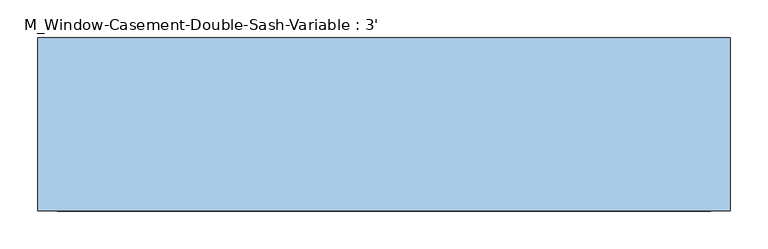
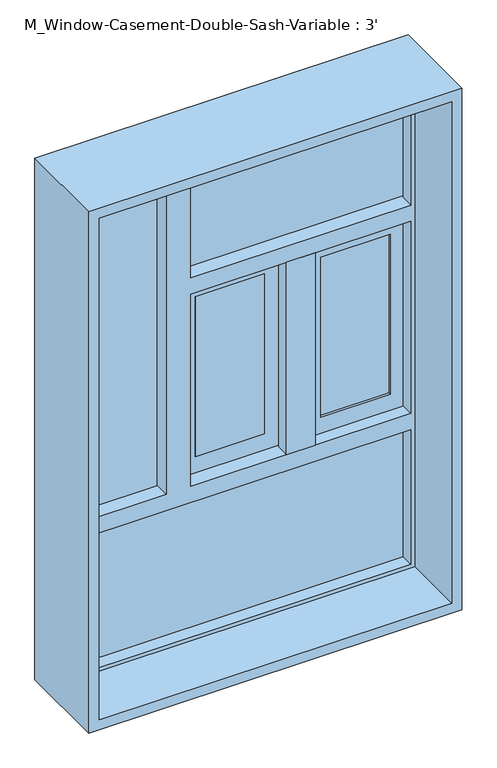
"""IFC4 building model written with IfcOpenShell, lengths in millimetres: window geometry, M_Window-Casement-Double-Sash-Variable : 3'."""

from ifc_helpers import new_model, si_unit, frame, origin, place, context, project, spatial, polyline, outline, extrude, faceted_brep, source, transform, mapped, element, save


def m_window_casement_double_sash_variable_3_661e274a(model_context):
    return source(origin(), model_context, "Body", "SolidModel", [
        extrude(outline(polyline([(389.8796875, 98.425), (389.8796875, 92.075), (219.7203125, 92.075), (219.7203125, 98.425), (389.8796875, 98.425)])), frame((0.0, 0.0, 1367.8804688), z_axis=(0.0, 0.0, 1.0), x_axis=(1.0, 0.0, 0.0)), (0.0, 0.0, 1.0), 414.2390625),
        extrude(outline(polyline([(389.8796875, 85.725), (389.8796875, 79.375), (219.7203125, 79.375), (219.7203125, 85.725), (389.8796875, 85.725)])), frame((0.0, 0.0, 1367.8804688), z_axis=(0.0, 0.0, 1.0), x_axis=(1.0, 0.0, 0.0)), (0.0, 0.0, 1.0), 414.2390625),
        extrude(outline(polyline([(85.0796875, 98.425), (85.0796875, 92.075), (-85.0796875, 92.075), (-85.0796875, 98.425), (85.0796875, 98.425)])), frame((0.0, 0.0, 1367.8804688), z_axis=(0.0, 0.0, 1.0), x_axis=(1.0, 0.0, 0.0)), (0.0, 0.0, 1.0), 414.2390625),
        extrude(outline(polyline([(85.0796875, 85.725), (85.0796875, 79.375), (-85.0796875, 79.375), (-85.0796875, 85.725), (85.0796875, 85.725)])), frame((0.0, 0.0, 1367.8804688), z_axis=(0.0, 0.0, 1.0), x_axis=(1.0, 0.0, 0.0)), (0.0, 0.0, 1.0), 414.2390625),
        extrude(outline(polyline([(-177.8, 98.425), (-177.8, 92.075), (-431.8, 92.075), (-431.8, 98.425), (-177.8, 98.425)])), frame((0.0, 0.0, 1325.9601563), z_axis=(0.0, 0.0, 1.0), x_axis=(1.0, 0.0, 0.0)), (0.0, 0.0, 1.0), 898.6398438),
        extrude(outline(polyline([(-177.8, 85.725), (-177.8, 79.375), (-431.8, 79.375), (-431.8, 85.725), (-177.8, 85.725)])), frame((0.0, 0.0, 1325.9601563), z_axis=(0.0, 0.0, 1.0), x_axis=(1.0, 0.0, 0.0)), (0.0, 0.0, 1.0), 898.6398438),
        extrude(outline(polyline([(177.8, 111.125), (177.8, 73.025), (187.9203125, 73.025), (187.9203125, 41.275), (116.8796875, 41.275), (116.8796875, 73.025), (127.0, 73.025), (127.0, 111.125), (177.8, 111.125)])), frame((0.0, 0.0, 1325.9601563), z_axis=(0.0, 0.0, 1.0), x_axis=(1.0, 0.0, 0.0)), (0.0, 0.0, 1.0), 498.0796875),
        extrude(outline(polyline([(431.8, 85.725), (431.8, 79.375), (-127.0, 79.375), (-127.0, 85.725), (431.8, 85.725)])), frame((0.0, 0.0, 1865.9601563), z_axis=(0.0, 0.0, 1.0), x_axis=(1.0, 0.0, 0.0)), (0.0, 0.0, 1.0), 358.6398438),
        extrude(outline(polyline([(431.8, 98.425), (431.8, 92.075), (-127.0, 92.075), (-127.0, 98.425), (431.8, 98.425)])), frame((0.0, 0.0, 1865.9601563), z_axis=(0.0, 0.0, 1.0), x_axis=(1.0, 0.0, 0.0)), (0.0, 0.0, 1.0), 358.6398438),
        extrude(outline(polyline([(431.8, 98.425), (431.8, 92.075), (-431.8, 92.075), (-431.8, 98.425), (431.8, 98.425)])), frame((0.0, 0.0, 925.4), z_axis=(0.0, 0.0, 1.0), x_axis=(1.0, 0.0, 0.0)), (0.0, 0.0, 1.0), 358.6398437),
        extrude(outline(polyline([(431.8, 85.725), (431.8, 79.375), (-431.8, 79.375), (-431.8, 85.725), (431.8, 85.725)])), frame((0.0, 0.0, 925.4), z_axis=(0.0, 0.0, 1.0), x_axis=(1.0, 0.0, 0.0)), (0.0, 0.0, 1.0), 358.6398437),
        faceted_brep([(-431.8, 73.025, 2224.6), (-431.8, 114.325, 2224.6), (431.8, 114.325, 2224.6), (431.8, 73.025, 2224.6), (-127.0, 73.025, 2224.6), (-127.0, 111.125, 2224.6), (-177.8, 111.125, 2224.6), (-177.8, 73.025, 2224.6), (-421.6796875, 41.275, 2214.4796875), (-421.6796875, 73.025, 2214.4796875), (-177.8, 73.025, 2214.4796875), (-177.8, 41.275, 2214.4796875), (421.6796875, 73.025, 2214.4796875), (421.6796875, 41.275, 2214.4796875), (-116.8796875, 41.275, 2214.4796875), (-116.8796875, 73.025, 2214.4796875), (-431.8, -114.3, 2224.6), (-431.8, 41.275, 2224.6), (431.8, 41.275, 2224.6), (431.8, -114.3, 2224.6), (-457.2, 114.325, 2250.0), (-457.2, -114.3, 2250.0), (457.2, -114.3, 2250.0), (457.2, 114.325, 2250.0), (431.8, 114.325, 925.4), (431.8, 73.025, 925.4), (431.8, 73.025, 1284.0398438), (431.8, 111.125, 1284.0398438), (431.8, 111.125, 1325.9601563), (431.8, 73.025, 1325.9601563), (431.8, 73.025, 1824.0398438), (431.8, 111.125, 1824.0398438), (431.8, 111.125, 1865.9601563), (431.8, 73.025, 1865.9601563), (421.6796875, 73.025, 1865.9601563), (421.6796875, 41.275, 1865.9601563), (421.6796875, 73.025, 935.5203125), (421.6796875, 41.275, 935.5203125), (421.6796875, 41.275, 1284.0398438), (421.6796875, 73.025, 1284.0398438), (421.6796875, 73.025, 1325.9601563), (421.6796875, 41.275, 1325.9601563), (421.6796875, 41.275, 1824.0398438), (421.6796875, 73.025, 1824.0398438), (431.8, 41.275, 925.4), (431.8, -114.3, 925.4), (457.2, -114.3, 900.0), (457.2, 114.325, 900.0), (-431.8, 114.325, 925.4), (-431.8, 73.025, 925.4), (-421.6796875, 73.025, 935.5203125), (-421.6796875, 41.275, 935.5203125), (-431.8, 41.275, 925.4), (-431.8, -114.3, 925.4), (-457.2, -114.3, 900.0), (-457.2, 114.325, 900.0), (-431.8, 73.025, 1325.9601563), (-431.8, 111.125, 1325.9601563), (-431.8, 111.125, 1284.0398438), (-431.8, 73.025, 1284.0398438), (-116.8796875, 73.025, 1865.9601563), (-127.0, 73.025, 1865.9601563), (-421.6796875, 73.025, 1284.0398438), (-421.6796875, 73.025, 1325.9601563), (-116.8796875, 73.025, 1325.9601563), (-127.0, 73.025, 1325.9601563), (-127.0, 73.025, 1824.0398438), (-116.8796875, 73.025, 1824.0398438), (-421.6796875, 41.275, 1325.9601563), (-421.6796875, 41.275, 1284.0398438), (-116.8796875, 41.275, 1865.9601563), (-177.8, 41.275, 1325.9601563), (-116.8796875, 41.275, 1325.9601563), (-116.8796875, 41.275, 1824.0398438), (-177.8, 111.125, 1325.9601563), (-127.0, 111.125, 1865.9601563), (-127.0, 111.125, 1824.0398438), (-127.0, 111.125, 1325.9601563)], [[[0, 1, 2, 3, 4, 5, 6, 7]], [[8, 9, 10, 11]], [[12, 13, 14, 15]], [[16, 17, 18, 19]], [[20, 21, 22, 23]], [[3, 2, 24, 25, 26, 27, 28, 29, 30, 31, 32, 33]], [[13, 12, 34, 35]], [[36, 37, 38, 39]], [[40, 41, 42, 43]], [[19, 18, 44, 45]], [[23, 22, 46, 47]], [[25, 24, 48, 49]], [[37, 36, 50, 51]], [[45, 44, 52, 53]], [[47, 46, 54, 55]], [[1, 0, 56, 57, 58, 59, 49, 48]], [[12, 15, 60, 61, 4, 3, 33, 34]], [[25, 49, 59, 62, 50, 36, 39, 26]], [[56, 0, 7, 10, 9, 63]], [[29, 40, 43, 30]], [[64, 65, 66, 67]], [[9, 8, 68, 63]], [[51, 50, 62, 69]], [[52, 44, 18, 17], [14, 13, 35, 70], [37, 51, 69, 38], [68, 8, 11, 71], [72, 73, 42, 41]], [[17, 16, 53, 52]], [[22, 21, 54, 46], [16, 19, 45, 53]], [[21, 20, 55, 54]], [[20, 23, 47, 55], [2, 1, 48, 24]], [[58, 27, 26, 39, 38, 69, 62, 59]], [[27, 58, 57, 74, 6, 5, 75, 32, 31, 76, 77, 28]], [[29, 28, 77, 65, 64, 72, 41, 40]], [[57, 56, 63, 68, 71, 74]], [[6, 74, 71, 11, 10, 7]], [[15, 14, 70, 60]], [[72, 64, 67, 73]], [[5, 4, 61, 75]], [[65, 77, 76, 66]], [[76, 31, 30, 43, 42, 73, 67, 66]], [[32, 75, 61, 60, 70, 35, 34, 33]]]),
        extrude(outline(polyline([(1824.0398438, 177.8), (1325.9601563, 177.8), (1325.9601563, 431.8), (1824.0398438, 431.8), (1824.0398438, 177.8)]), holes=[polyline([(1782.1195313, 389.8796875), (1367.8804688, 389.8796875), (1367.8804688, 219.7203125), (1782.1195313, 219.7203125), (1782.1195313, 389.8796875)])]), frame((0.0, 73.025, 0.0), z_axis=(0.0, 1.0, 0.0), x_axis=(0.0, 0.0, 1.0)), (0.0, 0.0, 1.0), 31.75),
        extrude(outline(polyline([(1824.0398438, -127.0), (1325.9601563, -127.0), (1325.9601563, 127.0), (1824.0398438, 127.0), (1824.0398438, -127.0)]), holes=[polyline([(1782.1195313, 85.0796875), (1367.8804688, 85.0796875), (1367.8804688, -85.0796875), (1782.1195313, -85.0796875), (1782.1195313, 85.0796875)])]), frame((0.0, 79.375, 0.0), z_axis=(0.0, 1.0, 0.0), x_axis=(0.0, 0.0, 1.0)), (0.0, 0.0, 1.0), 25.4),
    ])


if __name__ == "__main__":
    model = new_model("IFC4")
    model_context = context("Model", 3, world=origin())
    ifc_project = project(units=[si_unit("LENGTHUNIT", "METRE", prefix="MILLI")], contexts=[model_context])
    site = spatial("IfcSite", under=ifc_project)
    building = spatial("IfcBuilding", under=site)
    placement = place(None, origin())
    m_window_casement_double_sash_variable_3_shape = m_window_casement_double_sash_variable_3_661e274a(model_context)
    element("IfcWindow", 1, ObjectType="M_Window-Casement-Double-Sash-Variable : 3'", at=placement, inside=building, context=model_context, shape_type="MappedRepresentation", body=[
        mapped(m_window_casement_double_sash_variable_3_shape, transform((0.0, 0.0, 0.0), x_axis=(1.0, 0.0, 0.0), y_axis=(0.0, 1.0, 0.0), z_axis=(0.0, 0.0, 1.0))),
    ])
    save(model, "model.ifc")

# Revit data of these elements
# Type "M_Window-Casement-Double-Sash-Variable : 3'"
#   Type Mark = "36"
#   Fire Rating = "0.5h"
#   Assembly Code = "B2020100"
#   Analytic Construction = "Double glazing - domestic"
#   Window Inset [instance default] = 0' - 0 5/8"
#   Wall Thickness [instance default] = 0' - 5.90551"
#   Visual Light Transmittance = 0.81
#   Transom Height Ratio = 0.3
#   Transom Height = 1' - 3.94488"
#   Thermal Resistance (R) = 0.319569 (m²·K)/W
#   Solar Heat Gain Coefficient = 0.76
#   Rough Width = 3' - 0.59055"
#   Rough Height = 4' - 5.74016"
#   Opening Window Height = 1' - 9.25984"
#   Heat Transfer Coefficient (U) = 3.12929 W/(m²·K)
#   Height = 4' - 5.14961"
#   Frame Gap 3 [instance default] = 0' - 1.65041"
#   Frame Gap 2 [instance default] = 0' - 0.62598"
#   Frame Gap 1 = 0' - 1 51/128"
#   Window Width = 1' - 0"
#   Default Sill Height = 2' - 11.43307"
#   Width = 3' - 0"
#   Frame Material = Metal - Aluminum
#   Glass Panel Material = Glass
#   Wall Closure = (empty or 0)
# Element 1 (IfcWindow, "M_Window-Casement-Double-Sash-Variable : 3'")
#   Wall Thickness = 0' - 9"
#   Materials on its faces: "Metal - Aluminum", "Glass"
# Materials
#   "Metal - Aluminum": class "Metal", colour RGB 247 247 247, transparency 0
#   "Glass": class "Glass", colour RGB 0 128 192, transparency 0.9, Description = "Soda Lime Glass", Cost = 0
